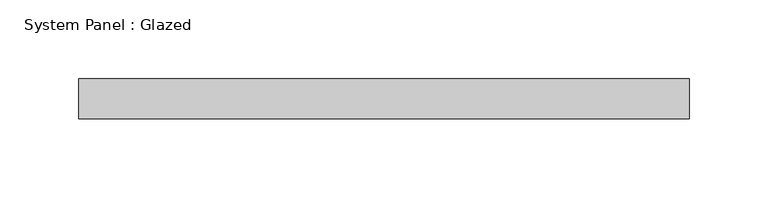
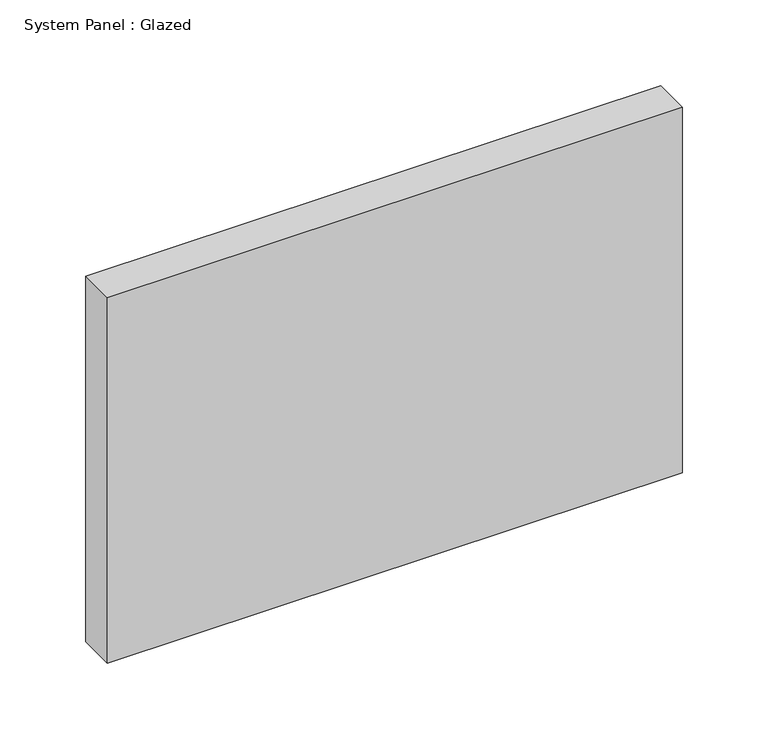
"""IFC4 building model written with IfcOpenShell, lengths in millimetres: plate geometry, System Panel : Glazed."""

from ifc_helpers import new_model, si_unit, origin, origin_with_axes, place, context, project, spatial, polyline, outline, extrude, source, transform, mapped, element, save


def system_panel_glazed_f9f57b5d(model_context):
    return source(origin(), model_context, "Body", "SweptSolid", [
        extrude(outline(polyline([(193.675, 19.05), (-193.675, 19.05), (-193.675, 44.45), (193.675, 44.45), (193.675, 19.05)])), origin_with_axes(), (0.0, 0.0, 1.0), 260.35),
    ])


if __name__ == "__main__":
    model = new_model("IFC4")
    model_context = context("Model", 3, world=origin())
    ifc_project = project(units=[si_unit("LENGTHUNIT", "METRE", prefix="MILLI")], contexts=[model_context])
    site = spatial("IfcSite", under=ifc_project)
    building = spatial("IfcBuilding", under=site)
    placement = place(None, origin())
    system_panel_glazed_shape = system_panel_glazed_f9f57b5d(model_context)
    element("IfcPlate", 1, ObjectType="System Panel : Glazed", at=placement, inside=building, context=model_context, shape_type="MappedRepresentation", body=[
        mapped(system_panel_glazed_shape, transform((0.0, 0.0, 0.0), x_axis=(1.0, 0.0, 0.0), y_axis=(0.0, 1.0, 0.0), z_axis=(0.0, 0.0, 1.0))),
    ])
    save(model, "model.ifc")

# Revit data of these elements
# Type "System Panel : Glazed"
#   Construction Type Id = "GSP4R"
#   Analytic Construction = "1/8 in Pilkington single glazing"
#   Visual Light Transmittance = 0.9
#   Solar Heat Gain Coefficient = 0.86
#   Heat Transfer Coefficient (U) = 1.18115 BTU/(h·ft²·°F)
#   Define Thermal Properties by = 1
# Element 1 (IfcPlate, "System Panel : Glazed")
#   Materials on its faces: "Glass"
# Materials
#   "Glass": class "Glass", colour RGB 0 128 192, transparency 0.75, Description = "Soda Lime Glass", Cost = 0
